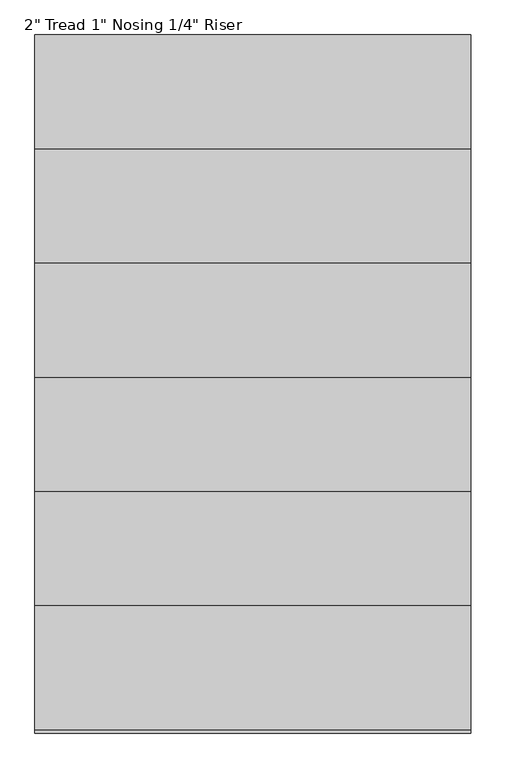
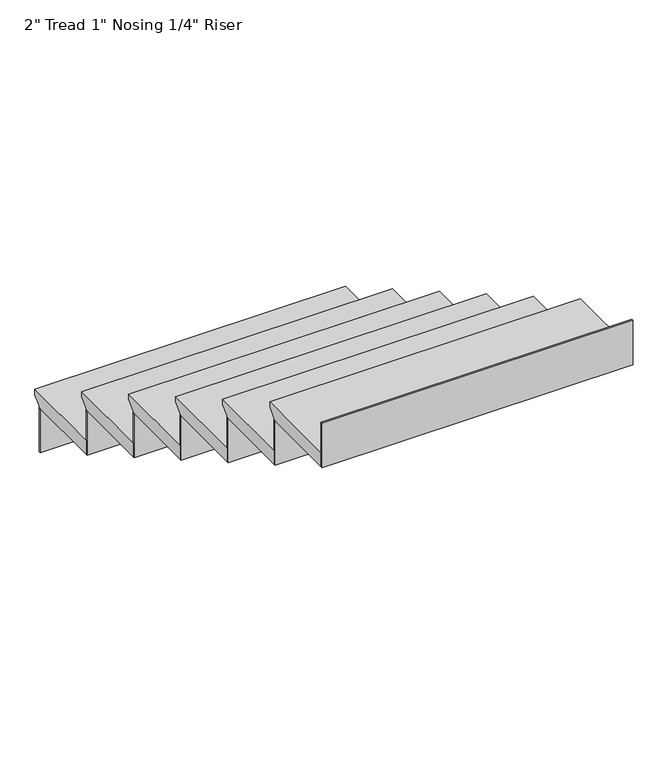
"""IFC4 building model written with IfcOpenShell, lengths in millimetres: stair flight geometry."""

from ifc_helpers import new_model, si_unit, frame, origin, place, context, project, spatial, polyline, outline, extrude, source, transform, mapped, element, save


def stair_flight_924b7841(model_context):
    return source(origin(), model_context, "Body", "SweptSolid", [
        extrude(outline(polyline([(4550.5468856, 2085.4736842), (4855.3468856, 2085.4736842), (4855.3468856, 2066.4236842), (4829.9468856, 2041.0236842), (4829.9468856, 2034.6736842), (4550.5468856, 2034.6736842), (4550.5468856, 2085.4736842)])), frame((-5084.5338869, 0.0, 0.0), z_axis=(1.0, 0.0, 0.0), x_axis=(0.0, 1.0, 0.0)), (0.0, 0.0, 1.0), 1066.8),
        extrude(outline(polyline([(-5084.5338869, 4823.5968856), (-5084.5338869, 4829.9468856), (-4017.7338869, 4829.9468856), (-4017.7338869, 4823.5968856), (-5084.5338869, 4823.5968856)])), frame((0.0, 0.0, 1874.2526316), z_axis=(0.0, 0.0, 1.0), x_axis=(1.0, 0.0, 0.0)), (0.0, 0.0, 1.0), 160.4210526),
        extrude(outline(polyline([(-5084.5338869, 4544.1968856), (-5084.5338869, 4550.5468856), (-4017.7338869, 4550.5468856), (-4017.7338869, 4544.1968856), (-5084.5338869, 4544.1968856)])), frame((0.0, 0.0, 2034.6736842), z_axis=(0.0, 0.0, 1.0), x_axis=(1.0, 0.0, 0.0)), (0.0, 0.0, 1.0), 160.4210526),
        extrude(outline(polyline([(4271.1468856, 2245.8947368), (4575.9468856, 2245.8947368), (4575.9468856, 2226.8447368), (4550.5468856, 2201.4447368), (4550.5468856, 2195.0947368), (4271.1468856, 2195.0947368), (4271.1468856, 2245.8947368)])), frame((-5084.5338869, 0.0, 0.0), z_axis=(1.0, 0.0, 0.0), x_axis=(0.0, 1.0, 0.0)), (0.0, 0.0, 1.0), 1066.8),
        extrude(outline(polyline([(-5084.5338869, 4264.7968856), (-5084.5338869, 4271.1468856), (-4017.7338869, 4271.1468856), (-4017.7338869, 4264.7968856), (-5084.5338869, 4264.7968856)])), frame((0.0, 0.0, 2195.0947368), z_axis=(0.0, 0.0, 1.0), x_axis=(1.0, 0.0, 0.0)), (0.0, 0.0, 1.0), 160.4210526),
        extrude(outline(polyline([(3991.7468856, 2406.3157895), (4296.5468856, 2406.3157895), (4296.5468856, 2387.2657895), (4271.1468856, 2361.8657895), (4271.1468856, 2355.5157895), (3991.7468856, 2355.5157895), (3991.7468856, 2406.3157895)])), frame((-5084.5338869, 0.0, 0.0), z_axis=(1.0, 0.0, 0.0), x_axis=(0.0, 1.0, 0.0)), (0.0, 0.0, 1.0), 1066.8),
        extrude(outline(polyline([(-5084.5338869, 3985.3968856), (-5084.5338869, 3991.7468856), (-4017.7338869, 3991.7468856), (-4017.7338869, 3985.3968856), (-5084.5338869, 3985.3968856)])), frame((0.0, 0.0, 2355.5157895), z_axis=(0.0, 0.0, 1.0), x_axis=(1.0, 0.0, 0.0)), (0.0, 0.0, 1.0), 160.4210526),
        extrude(outline(polyline([(3712.3468856, 2566.7368421), (4017.1468856, 2566.7368421), (4017.1468856, 2547.6868421), (3991.7468856, 2522.2868421), (3991.7468856, 2515.9368421), (3712.3468856, 2515.9368421), (3712.3468856, 2566.7368421)])), frame((-5084.5338869, 0.0, 0.0), z_axis=(1.0, 0.0, 0.0), x_axis=(0.0, 1.0, 0.0)), (0.0, 0.0, 1.0), 1066.8),
        extrude(outline(polyline([(-5084.5338869, 3705.9968856), (-5084.5338869, 3712.3468856), (-4017.7338869, 3712.3468856), (-4017.7338869, 3705.9968856), (-5084.5338869, 3705.9968856)])), frame((0.0, 0.0, 2515.9368421), z_axis=(0.0, 0.0, 1.0), x_axis=(1.0, 0.0, 0.0)), (0.0, 0.0, 1.0), 160.4210526),
        extrude(outline(polyline([(3432.9468856, 2727.1578947), (3737.7468856, 2727.1578947), (3737.7468856, 2708.1078947), (3712.3468856, 2682.7078947), (3712.3468856, 2676.3578947), (3432.9468856, 2676.3578947), (3432.9468856, 2727.1578947)])), frame((-5084.5338869, 0.0, 0.0), z_axis=(1.0, 0.0, 0.0), x_axis=(0.0, 1.0, 0.0)), (0.0, 0.0, 1.0), 1066.8),
        extrude(outline(polyline([(-5084.5338869, 3426.5968856), (-5084.5338869, 3432.9468856), (-4017.7338869, 3432.9468856), (-4017.7338869, 3426.5968856), (-5084.5338869, 3426.5968856)])), frame((0.0, 0.0, 2676.3578947), z_axis=(0.0, 0.0, 1.0), x_axis=(1.0, 0.0, 0.0)), (0.0, 0.0, 1.0), 160.4210526),
        extrude(outline(polyline([(-5084.5338869, 3147.1968856), (-5084.5338869, 3153.5468856), (-4017.7338869, 3153.5468856), (-4017.7338869, 3147.1968856), (-5084.5338869, 3147.1968856)])), frame((0.0, 0.0, 2836.7789474), z_axis=(0.0, 0.0, 1.0), x_axis=(1.0, 0.0, 0.0)), (0.0, 0.0, 1.0), 160.4210526),
        extrude(outline(polyline([(3153.5468856, 2887.5789474), (3458.3468856, 2887.5789474), (3458.3468856, 2868.5289474), (3432.9468856, 2843.1289474), (3432.9468856, 2836.7789474), (3153.5468856, 2836.7789474), (3153.5468856, 2887.5789474)])), frame((-5084.5338869, 0.0, 0.0), z_axis=(1.0, 0.0, 0.0), x_axis=(0.0, 1.0, 0.0)), (0.0, 0.0, 1.0), 1066.8),
    ])


if __name__ == "__main__":
    model = new_model("IFC4")
    model_context = context("Model", 3, world=origin())
    ifc_project = project(units=[si_unit("LENGTHUNIT", "METRE", prefix="MILLI")], contexts=[model_context])
    site = spatial("IfcSite", under=ifc_project)
    building = spatial("IfcBuilding", under=site)
    placement = place(None, origin())
    stair_flight_shape = stair_flight_924b7841(model_context)
    element("IfcStairFlight", 1, ObjectType="2\" Tread 1\" Nosing 1/4\" Riser", at=placement, inside=building, context=model_context, shape_type="MappedRepresentation", body=[
        mapped(stair_flight_shape, transform((0.0, 0.0, 0.0), x_axis=(1.0, 0.0, 0.0), y_axis=(0.0, 1.0, 0.0), z_axis=(0.0, 0.0, 1.0))),
    ])
    save(model, "model.ifc")
